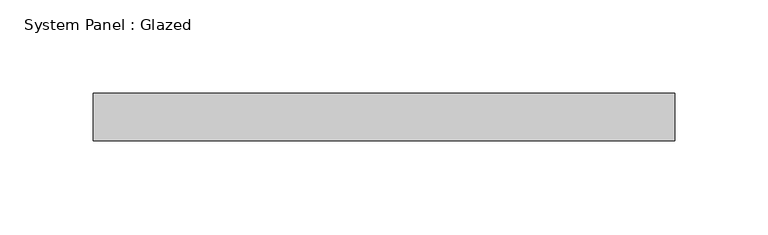
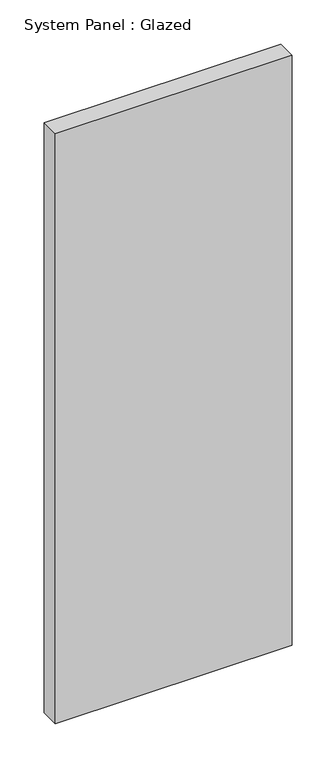
"""IFC4 building model written with IfcOpenShell, lengths in millimetres: plate geometry, System Panel : Glazed."""

from ifc_helpers import new_model, si_unit, origin, origin_with_axes, place, context, project, spatial, polyline, outline, extrude, source, transform, mapped, element, save


def system_panel_glazed_2f2cf5d5(model_context):
    return source(origin(), model_context, "Body", "SweptSolid", [
        extrude(outline(polyline([(155.575, 19.05), (-155.575, 19.05), (-155.575, 44.45), (155.575, 44.45), (155.575, 19.05)])), origin_with_axes(), (0.0, 0.0, 1.0), 818.8480012),
    ])


if __name__ == "__main__":
    model = new_model("IFC4")
    model_context = context("Model", 3, world=origin())
    ifc_project = project(units=[si_unit("LENGTHUNIT", "METRE", prefix="MILLI")], contexts=[model_context])
    site = spatial("IfcSite", under=ifc_project)
    building = spatial("IfcBuilding", under=site)
    placement = place(None, origin())
    system_panel_glazed_shape = system_panel_glazed_2f2cf5d5(model_context)
    element("IfcPlate", 1, ObjectType="System Panel : Glazed", at=placement, inside=building, context=model_context, shape_type="MappedRepresentation", body=[
        mapped(system_panel_glazed_shape, transform((0.0, 0.0, 0.0), x_axis=(1.0, 0.0, 0.0), y_axis=(0.0, 1.0, 0.0), z_axis=(0.0, 0.0, 1.0))),
    ])
    save(model, "model.ifc")

# Revit data of these elements
# Type "System Panel : Glazed"
#   Construction Type Id = "GSP4R"
#   Analytic Construction = "1/8 in Pilkington single glazing"
#   Visual Light Transmittance = 0.9
#   Solar Heat Gain Coefficient = 0.86
#   Heat Transfer Coefficient (U) = 1.18115 BTU/(h·ft²·°F)
# Element 1 (IfcPlate, "System Panel : Glazed")
#   Materials on its faces: "Glass"
# Materials
#   "Glass": class "Glass", colour RGB 0 128 192, transparency 0.75, Description = "Soda Lime Glass", Cost = 0
